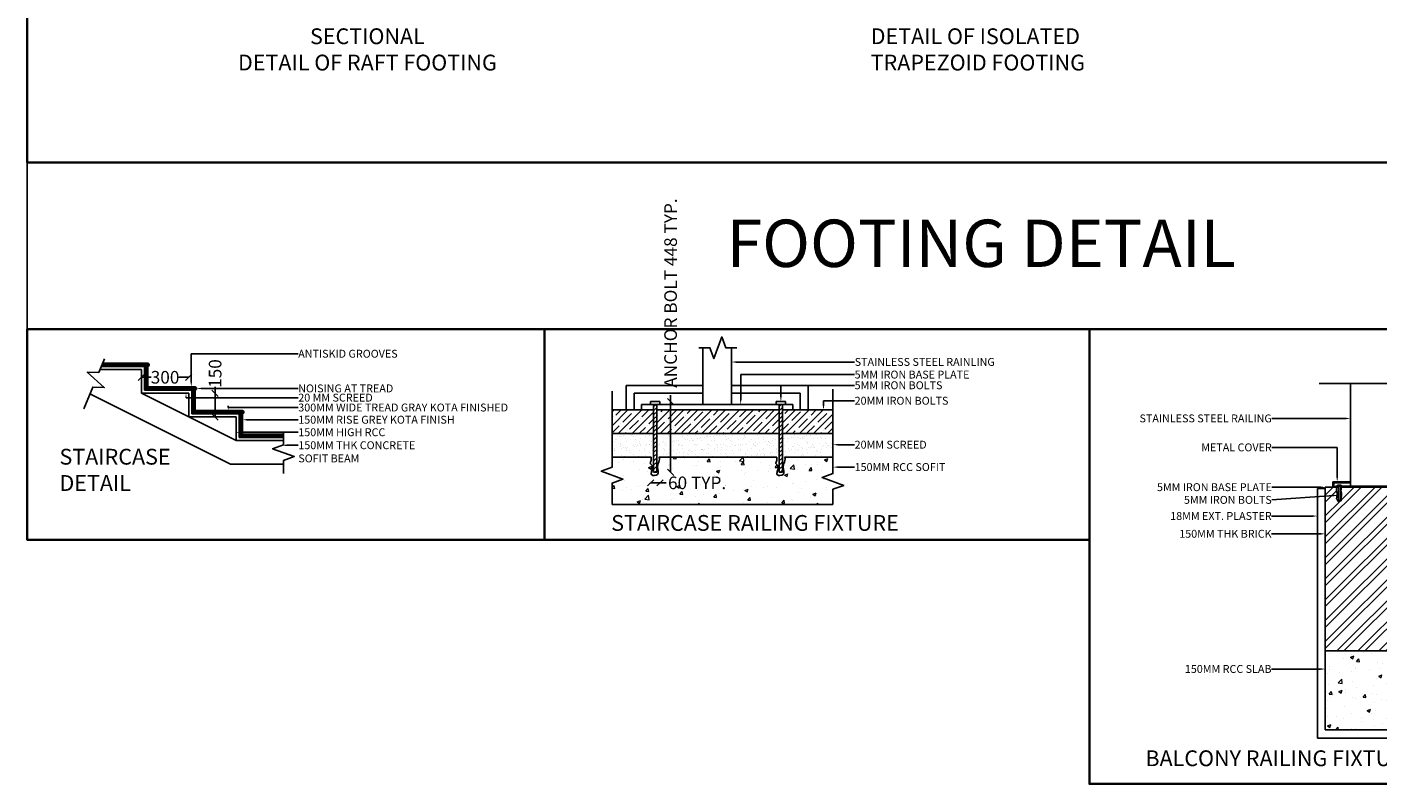
# Model space of a CAD drawing. Units: millimetres. Extents: x -6233 to 6805, y -5269 to 4890.
# Tile 1 of 4: x -6233 to 2321, y -5269 to -472. Entities that reach past the tile are written whole.
import ezdxf
from ezdxf import colors
from ezdxf.entities.mleader import LeaderData, LeaderLine
from ezdxf.math import Vec2, Vec3

# ---------------------------------------------------------------- set-up
doc = ezdxf.new("R2010")
doc.units = ezdxf.units.MM
doc.header["$MEASUREMENT"] = 0
for name, color, linetype, lineweight in [('A-FLOR-HRAL', 4, 'Continuous', 25), ('A-FLOR-STRS', 7, 'Continuous', 25), ('S-ANNO-DIMS', 2, 'Continuous', 18), ('S-ANNO-TEXT', 3, 'Continuous', 18), ('S-ANNO-TTLB', 7, 'Continuous', 35), ('S-PATT', 252, 'Continuous', 13)]:
    doc.layers.add(name, color=color, linetype=linetype, lineweight=lineweight)
doc.styles.get("Standard").update_dxf_attribs({"font": 'arial.ttf'})
doc.dimstyles.get("Standard").update_dxf_attribs({"dimtxt": 80, "dimasz": 40, "dimexe": 0.18, "dimexo": 0.0625, "dimgap": 0.09, "dimtad": 0, "dimdec": 0, "dimzin": 0, "dimdsep": 46, "dimtxsty": 'Standard', "dimblk": 'OBLIQUE', "dimcen": 0.09, "dimadec": 0, "dimazin": 0, "dimtfac": 1, "dimtdec": 0, "dimtofl": 0, "dimtmove": 0, "dimatfit": 3, "dimfxl": 1, "dimfxlon": 1, "dimtolj": 1, "dimtzin": 0, "dimarcsym": 0})

# ---------------------------------------------------------------- blocks, each defined once
blk = doc.blocks.new('_Oblique')
at = {"color": 0, "linetype": 'ByBlock', "lineweight": -2}
blk.add_line((-0.5, -0.5), (0.5, 0.5), dxfattribs=at)
blk = doc.blocks.new('*D23')
at = {"layer": 'DEFPOINTS', "color": 0, "transparency": 16777216}
for p in [(-5208.1, -2691.9), (-5508.1, -2792.8), (-5208.1, -2792.8)]:
    blk.add_point(p, dxfattribs=at)
at = {"layer": 'S-ANNO-DIMS', "color": 0, "lineweight": -2, "transparency": 16777216}
for p, q in [((-5508.1, -2692.9), (-5508.1, -2691.7)), ((-5508.1, -2691.9), (-5446.4, -2691.9)), ((-5208.1, -2691.9), (-5269.8, -2691.9)), ((-5208.1, -2692.9), (-5208.1, -2691.7))]:
    blk.add_line(p, q, dxfattribs=at)
at = {"layer": 'S-ANNO-DIMS', "color": 0, "lineweight": -2, "transparency": 16777216, "xscale": 40, "yscale": 40, "zscale": 40, "rotation": 180}
blk.add_blockref('_Oblique', (-5508.1, -2691.9), dxfattribs=at)
at = {"layer": 'S-ANNO-DIMS', "color": 0, "lineweight": -2, "transparency": 16777216, "xscale": 40, "yscale": 40, "zscale": 40}
blk.add_blockref('_Oblique', (-5208.1, -2691.9), dxfattribs=at)
at = {"layer": 'S-ANNO-DIMS', "color": 0, "transparency": 16777216, "insert": (-5358.1, -2691.9), "char_height": 80, "attachment_point": 5}
blk.add_mtext('\\A1;300', dxfattribs=at)
blk = doc.blocks.new('*D24')
at = {"layer": 'DEFPOINTS', "color": 0, "transparency": 16777216}
for p in [(-5208.1, -2792.8), (-5040.8, -2792.8), (-5208.1, -2942.8)]:
    blk.add_point(p, dxfattribs=at)
at = {"layer": 'S-ANNO-DIMS', "color": 0, "lineweight": -2, "transparency": 16777216}
for p, q in [((-5041.8, -2792.8), (-5040.6, -2792.8)), ((-5040.8, -2792.8), (-5040.8, -2752.8)), ((-5040.8, -2942.8), (-5040.8, -2792.8)), ((-5041.8, -2942.8), (-5040.6, -2942.8))]:
    blk.add_line(p, q, dxfattribs=at)
at = {"layer": 'S-ANNO-DIMS', "color": 0, "lineweight": -2, "transparency": 16777216, "xscale": 40, "yscale": 40, "zscale": 40}
for p, rotation in [((-5040.8, -2792.8), 90), ((-5040.8, -2942.8), 270)]:
    blk.add_blockref('_Oblique', p, dxfattribs=dict(at, rotation=rotation))
at = {"layer": 'S-ANNO-DIMS', "color": 0, "transparency": 16777216, "insert": (-5040.8, -2668.2), "char_height": 80, "attachment_point": 5, "rotation": 90}
blk.add_mtext('\\A1;150', dxfattribs=at)
blk = doc.blocks.new('ANCHOR-BOLT-STAIR')
for p, q in [((0, 429.2), (0, 447.9)), ((0, 447.9), (59.9, 447.9)), ((19.4, 429.2), (0, 429.2)), ((19.4, 429.2), (19.4, 0)), ((39.4, 429.2), (39.4, 0)), ((59.9, 429.2), (39.4, 429.2)), ((59.9, 447.9), (59.9, 429.2)), ((39.4, 0), (19.4, 0))]:
    blk.add_line(p, q)
blk = doc.blocks.new('*D32')
at = {"layer": 'DEFPOINTS', "color": 0, "transparency": 16777216}
for p in [(-2222, -2845.6), (-2154.8, -2845.6), (-2222, -3293.5)]:
    blk.add_point(p, dxfattribs=at)
at = {"layer": 'S-ANNO-DIMS', "color": 0, "lineweight": -2, "transparency": 16777216}
for p, q in [((-2154.8, -2845.6), (-2154.8, -2805.6)), ((-2155.8, -2845.6), (-2154.7, -2845.6)), ((-2154.8, -3293.5), (-2154.8, -2845.6)), ((-2155.8, -3293.5), (-2154.7, -3293.5))]:
    blk.add_line(p, q, dxfattribs=at)
at = {"layer": 'S-ANNO-DIMS', "color": 0, "lineweight": -2, "transparency": 16777216, "xscale": 40, "yscale": 40, "zscale": 40}
for p, rotation in [((-2154.8, -2845.6), 90), ((-2154.8, -3293.5), 270)]:
    blk.add_blockref('_Oblique', p, dxfattribs=dict(at, rotation=rotation))
at = {"layer": 'S-ANNO-DIMS', "color": 0, "transparency": 16777216, "insert": (-2154.8, -2158.3), "char_height": 80, "attachment_point": 5, "rotation": 90}
blk.add_mtext('\\A1;ANCHOR BOLT 448 TYP.', dxfattribs=at)
blk = doc.blocks.new('*D33')
at = {"layer": 'DEFPOINTS', "color": 0, "transparency": 16777216}
for p in [(-2281.9, -3293.5), (-2222, -3293.5), (-2222, -3360.7)]:
    blk.add_point(p, dxfattribs=at)
at = {"layer": 'S-ANNO-DIMS', "color": 0, "lineweight": -2, "transparency": 16777216}
for p, q in [((-2281.9, -3359.7), (-2281.9, -3360.8)), ((-2281.9, -3360.7), (-2222, -3360.7)), ((-2222, -3359.7), (-2222, -3360.8)), ((-2222, -3360.7), (-2182, -3360.7))]:
    blk.add_line(p, q, dxfattribs=at)
at = {"layer": 'S-ANNO-DIMS', "color": 0, "lineweight": -2, "transparency": 16777216, "xscale": 40, "yscale": 40, "zscale": 40, "rotation": 180}
blk.add_blockref('_Oblique', (-2281.9, -3360.7), dxfattribs=at)
at = {"layer": 'S-ANNO-DIMS', "color": 0, "lineweight": -2, "transparency": 16777216, "xscale": 40, "yscale": 40, "zscale": 40}
blk.add_blockref('_Oblique', (-2222, -3360.7), dxfattribs=at)
at = {"layer": 'S-ANNO-DIMS', "color": 0, "transparency": 16777216, "insert": (-1987, -3360.7), "char_height": 80, "attachment_point": 5}
blk.add_mtext('\\A1;60 TYP.', dxfattribs=at)

msp = doc.modelspace()

# ---------------------------------------------------------------- hatches: boundary and pattern name
at = {"layer": 'S-PATT'}
h = msp.add_hatch(dxfattribs=at)
h.set_pattern_fill('ANSI31', color=256, scale=50)
h.set_pattern_definition([(45, (445.642, 4418.545), (-4.4194174, 4.4194174), [])])
h.paths.add_polyline_path([(-5468.1, -2602.8), (-5753.6, -2602.8), (-5761.9, -2622.8), (-5468.1, -2622.8, 1)])
h.paths.add_polyline_path([(-5468.1, -2622.8), (-5488.1, -2622.8), (-5488.1, -2772.8), (-5168.1, -2772.8, 1), (-5168.1, -2752.8), (-5468.1, -2752.8)])
h.paths.add_polyline_path([(-5168.1, -2772.8), (-5188.1, -2772.8), (-5188.1, -2922.8), (-4868.1, -2922.8, 1), (-4868.1, -2902.8), (-5168.1, -2902.8)])
h.paths.add_polyline_path([(-4868.1, -2922.8), (-4888.1, -2922.8), (-4888.1, -3072.8), (-4608.1, -3072.8), (-4608.1, -3052.8), (-4868.1, -3052.8)])
h = msp.add_hatch(dxfattribs=at)
h.set_pattern_fill('ANSI35', color=256, scale=250)
h.set_pattern_definition([(45, (1728.94, 2227.43), (-44.1942, 44.1942), []), (45, (1773.14, 2227.43), (-44.1942, 44.1942), [78.125, -15.625, 0, -15.625])])
h.paths.add_polyline_path([(-1466.5, -2898.6), (-2242.5, -2898.6), (-2242.5, -3048.6), (-1466.5, -3048.6)])
h.paths.add_polyline_path([(-1126.1, -2898.6), (-1446.5, -2898.6), (-1446.5, -3048.6), (-1126.1, -3048.6)])
h.paths.add_polyline_path([(-2262.5, -2898.6), (-2525.7, -2898.6), (-2525.7, -3048.6), (-2262.5, -3048.6)])
h = msp.add_hatch(dxfattribs=at)
h.set_pattern_fill('ANSI31', color=256, scale=150)
h.set_pattern_definition([(45, (1728.943, 2227.432), (-13.25825, 13.25825), [])])
h.paths.add_polyline_path([(-2242.5, -2864.2), (-2262.5, -2864.2), (-2262.5, -3293.5), (-2242.5, -3293.5)])
h.paths.add_polyline_path([(-1446.5, -2864.2), (-1466.5, -2864.2), (-1466.5, -3293.5), (-1446.5, -3293.5)])
h = msp.add_hatch(dxfattribs=at)
h.set_pattern_fill('AR-SAND', color=256, scale=30)
h.set_pattern_definition([(37.5, (1728.943, 2227.43), (-1.8898, 57.8047), [0, -45.6, 0, -51, 0, -48.75]), (7.5, (1728.94, 2227.43), (53.0933, 84.6644), [0, -24.6, 0, -41.1, 0, -15.75]), (327.5, (1692.043, 2227.43), (93.42426, 0.16977), [0, -15, 0, -54, 0, -70.5]), (317.5, (1692.04, 2227.43), (90.1838, 26.3303), [0, -7.5, 0, -35.4, 0, -40.5])])
edge = h.paths.add_edge_path()
edge.add_line((-1466.5, -3048.6), (-2242.5, -3048.6))
edge.add_line((-2242.5, -3048.6), (-2242.5, -3293.5))
edge.add_line((-2242.5, -3293.5), (-2262.5, -3293.5))
edge.add_line((-2262.5, -3293.5), (-2262.5, -3048.6))
edge.add_line((-2262.5, -3048.6), (-2525.7, -3048.6))
edge.add_line((-2525.7, -3048.6), (-2525.7, -3198.6))
edge.add_line((-2525.7, -3198.6), (-2278.6, -3198.6))
edge.add_spline(control_points=[(-2278.6, -3198.6), (-2277.5, -3205.6), (-2275.5, -3218.5), (-2288.7, -3238.2), (-2260.8, -3253.8), (-2274.9, -3281.2), (-2280.9, -3317.9), (-2219.2, -3315.1), (-2245.1, -3262.2), (-2230.5, -3234.1), (-2221.5, -3202.7), (-2229.8, -3198.6)], knot_values=[0, 0, 0, 0, 20.99677, 39.349881, 56.133346, 95.091284, 114.829491, 151.719513, 198.433264, 232.426652, 262.634584, 262.634584, 262.634584, 262.634584], degree=3, periodic=0)
edge.add_line((-2229.8, -3198.6), (-1482.5, -3198.6))
edge.add_spline(control_points=[(-1482.5, -3198.6), (-1481.5, -3205.6), (-1479.5, -3218.5), (-1492.6, -3238.2), (-1464.8, -3253.8), (-1478.9, -3281.2), (-1484.9, -3317.9), (-1423.2, -3315.1), (-1449.1, -3262.2), (-1434.4, -3234.1), (-1425.5, -3202.7), (-1433.8, -3198.6)], knot_values=[0, 0, 0, 0, 20.99677, 39.349881, 56.133346, 95.091284, 114.829491, 151.719513, 198.433264, 232.426652, 262.634584, 262.634584, 262.634584, 262.634584], degree=3, periodic=0)
edge.add_line((-1433.8, -3198.6), (-1126.1, -3198.6))
edge.add_line((-1126.1, -3198.6), (-1126.1, -3048.6))
edge.add_line((-1126.1, -3048.6), (-1446.5, -3048.6))
edge.add_line((-1446.5, -3048.6), (-1446.5, -3293.5))
edge.add_line((-1446.5, -3293.5), (-1466.5, -3293.5))
edge.add_line((-1466.5, -3293.5), (-1466.5, -3048.6))
h = msp.add_hatch(dxfattribs=at)
h.set_pattern_fill('AR-CONC', color=256, scale=30)
h.set_pattern_definition([(50, (1728.94, 2227.43), (215.178, -18.8256), [22.5, -247.5]), (355, (1728.94, 2227.43), (-41.6254, 225.6576), [18, -198]), (100.4514, (1746.87, 2225.86), (173.5527, 206.832), [19.122, -210.3426]), (46.184, (1728.94, 2287.43), (320.172, -49.656), [33.75, -371.25]), (96.6356, (1755.62, 2283.3), (280.399, 292.236), [28.683, -315.514]), (351.184, (1728.94, 2287.43), (280.399, 292.236), [27, -297]), (21, (1758.94, 2272.43), (179.072, -120.7857), [22.5, -247.5]), (326, (1758.94, 2272.43), (72.9946, 217.545), [18, -198]), (71.4514, (1773.87, 2262.37), (252.067, 96.7593), [19.122, -210.3426]), (37.5, (1728.94, 2227.43), (3.64796, 99.86816), [0, -195.6, 0, -201, 0, -198.75]), (7.5, (1728.94, 2227.43), (78.9209, 118.3235), [0, -114.6, 0, -191.1, 0, -75.75]), (327.5, (1662.04, 2227.43), (160.1467, -6.7665), [0, -75, 0, -234, 0, -310.5]), (317.5, (1632.04, 2227.43), (174.9559, 30.0315), [0, -97.5, 0, -155.4, 0, -220.5])])
edge = h.paths.add_edge_path()
edge.add_spline(control_points=[(-2229.8, -3198.6), (-2221.5, -3202.7), (-2230.5, -3234.1), (-2245.1, -3262.2), (-2219.2, -3315.1), (-2280.9, -3317.9), (-2274.9, -3281.2), (-2260.8, -3253.8), (-2288.7, -3238.2), (-2275.5, -3218.5), (-2277.5, -3205.6), (-2278.6, -3198.6)], knot_values=[0, 0, 0, 0, 30.207932, 64.20132, 110.915071, 147.805093, 167.5433, 206.501238, 223.284703, 241.637814, 262.634584, 262.634584, 262.634584, 262.634584], degree=3, periodic=0)
edge.add_line((-2278.6, -3198.6), (-2525.7, -3198.6))
edge.add_line((-2525.7, -3198.6), (-2525.7, -3262.3))
edge.add_line((-2525.7, -3262.3), (-2594.4, -3287.3))
edge.add_line((-2594.4, -3287.3), (-2457, -3337.3))
edge.add_line((-2457, -3337.3), (-2525.7, -3362.3))
edge.add_line((-2525.7, -3362.3), (-2525.7, -3498.6))
edge.add_line((-2525.7, -3498.6), (-1126.1, -3498.6))
edge.add_line((-1126.1, -3498.6), (-1126.1, -3401.8))
edge.add_line((-1126.1, -3401.8), (-1057.5, -3376.8))
edge.add_line((-1057.5, -3376.8), (-1194.8, -3326.8))
edge.add_line((-1194.8, -3326.8), (-1126.1, -3301.8))
edge.add_line((-1126.1, -3301.8), (-1126.1, -3198.6))
edge.add_line((-1126.1, -3198.6), (-1433.8, -3198.6))
edge.add_spline(control_points=[(-1433.8, -3198.6), (-1425.5, -3202.7), (-1434.4, -3234.1), (-1449.1, -3262.2), (-1423.2, -3315.1), (-1484.9, -3317.9), (-1478.9, -3281.2), (-1464.8, -3253.8), (-1492.6, -3238.2), (-1479.5, -3218.5), (-1481.5, -3205.6), (-1482.5, -3198.6)], knot_values=[0, 0, 0, 0, 30.207932, 64.20132, 110.915071, 147.805093, 167.5433, 206.501238, 223.284703, 241.637814, 262.634584, 262.634584, 262.634584, 262.634584], degree=3, periodic=0)
edge.add_line((-1482.5, -3198.6), (-2229.8, -3198.6))
h = msp.add_hatch(dxfattribs=at)
h.set_pattern_fill('ANSI32', color=256, scale=250)
h.set_pattern_definition([(45, (-403.88, 395.55), (-66.2913, 66.2913), []), (45, (-359.68, 395.55), (-66.2913, 66.2913), [])])
h.paths.add_polyline_path([(2555.6, -3388.6), (2479.2, -3388.6), (2475, -3412), (2479.2, -3425.9), (2479.2, -3442.8), (2477.2, -3451.1), (2477.2, -3475.2), (2457.7, -3479.6), (2450.6, -3467.1), (2447.4, -3461.6), (2448.4, -3451.9), (2451.4, -3421.4), (2447.5, -3414.8), (2447.5, -3401.8), (2448.7, -3388.6), (2096.7, -3388.6), (2092.6, -3412), (2096.7, -3425.9), (2096.7, -3442.8), (2094.8, -3451), (2094.8, -3475.2), (2075.3, -3479.6), (2068.2, -3467.1), (2065, -3461.6), (2065.9, -3451.9), (2069, -3421.4), (2065.1, -3414.8), (2065.1, -3401.8), (2066.2, -3388.6), (1993.8, -3388.6), (1993.8, -4425), (2555.6, -4425)])
h = msp.add_hatch(dxfattribs=at)
h.set_pattern_fill('AR-CONC', color=256, scale=30)
h.set_pattern_definition([(50, (-403.88, 395.55), (215.178, -18.8256), [22.5, -247.5]), (355, (-403.88, 395.55), (-41.6254, 225.658), [18, -198]), (100.4514, (-385.94, 393.99), (173.5527, 206.832), [19.122, -210.3426]), (46.184, (-403.88, 455.55), (320.172, -49.656), [33.75, -371.25]), (96.6356, (-377.2, 451.42), (280.399, 292.236), [28.683, -315.514]), (351.184, (-403.88, 455.55), (280.399, 292.236), [27, -297]), (21, (-373.88, 440.55), (179.072, -120.7857), [22.5, -247.5]), (326, (-373.88, 440.55), (72.9946, 217.545), [18, -198]), (71.4514, (-358.95, 430.49), (252.067, 96.7593), [19.122, -210.3426]), (37.5, (-403.88, 395.554), (3.648, 99.8682), [0, -195.6, 0, -201, 0, -198.75]), (7.5, (-403.88, 395.55), (78.9209, 118.3235), [0, -114.6, 0, -191.1, 0, -75.75]), (327.5, (-470.78, 395.55), (160.1467, -6.7665), [0, -75, 0, -234, 0, -310.5]), (317.5, (-500.78, 395.55), (174.9559, 30.0315), [0, -97.5, 0, -155.4, 0, -220.5])])
h.paths.add_polyline_path([(3117.4, -4925), (3117.4, -4675), (3460.8, -4550), (3117.4, -4425), (1993.8, -4425), (1993.8, -4925)])

# ---------------------------------------------------------------- linework, layer by layer
at = {"layer": 'A-FLOR-HRAL'}
for p, q in [((-1951, -2864.2), (-1951, -2505.1)), ((-1769.2, -2864.2), (-1769.2, -2505.1)), ((2153.7, -3388.6), (2153.7, -2730.5)), ((-2436, -2898.6), (-2436, -2743)), ((-2436, -2743), (-1951, -2743)), ((-2386, -2898.6), (-2386, -2793)), ((-2386, -2793), (-1951, -2793)), ((-1284.2, -2743), (-1769.2, -2743)), ((-1334.2, -2793), (-1769.2, -2793)), ((-1334.2, -2898.6), (-1334.2, -2793)), ((-1284.2, -2898.6), (-1284.2, -2743)), ((-2525.7, -2898.6), (-2262.5, -2898.6)), ((-2525.7, -2898.6), (-2262.5, -2898.6)), ((-1380.8, -2864.2), (-2339.4, -2864.2)), ((-2339.4, -2864.2), (-2339.4, -2898.6)), ((-2242.5, -2898.6), (-1466.5, -2898.6)), ((-2242.5, -2898.6), (-1466.5, -2898.6)), ((-1446.5, -2898.6), (-1126.1, -2898.6)), ((-1446.5, -2898.6), (-1126.1, -2898.6)), ((-1380.8, -2898.6), (-1380.8, -2864.2)), ((-2525.7, -3048.6), (-2262.5, -3048.6)), ((-2242.5, -3048.6), (-1466.5, -3048.6)), ((-1446.5, -3048.6), (-1126.1, -3048.6)), ((-2525.7, -3198.6), (-2278.6, -3198.6)), ((-2229.8, -3198.6), (-1482.5, -3198.6)), ((-1433.8, -3198.6), (-1126.1, -3198.6)), ((1993.8, -3397.4), (1943.8, -3397.4)), ((1943.8, -3397.4), (1943.8, -4979.4)), ((1993.8, -3388.6), (1993.8, -4925)), ((1993.8, -3388.6), (2077.2, -3388.6)), ((2077.2, -3388.6), (1993.8, -3388.6)), ((2042.3, -3388.6), (2042.3, -3355.2)), ((2042.3, -3355.2), (2153.7, -3355.2)), ((2048.2, -3388.6), (2048.2, -3359.8)), ((2048.2, -3359.8), (2153.7, -3359.8)), ((2486.4, -3382.1), (2057.2, -3382.1)), ((2057.2, -3382.1), (2057.2, -3388.6)), ((2066.2, -3388.6), (2065.1, -3401.8)), ((2065.1, -3401.8), (2065.1, -3414.8)), ((2065.1, -3414.8), (2069, -3421.4)), ((2069, -3421.4), (2065.9, -3451.9)), ((2094.2, -3376), (2071.7, -3376)), ((2071.7, -3376), (2071.7, -3382.1)), ((2071.7, -3382.1), (2075.5, -3382.1)), ((2088, -3382.1), (2075.5, -3382.1)), ((2077.2, -3382.1), (2077.2, -3472.8)), ((2088, -3382.1), (2094.2, -3382.1)), ((2089.6, -3472.8), (2089.6, -3382.1)), ((2089.6, -3388.6), (2459.7, -3388.6)), ((2459.7, -3388.6), (2089.6, -3388.6)), ((2092.6, -3412), (2096.7, -3388.6)), ((2096.7, -3425.9), (2092.6, -3412)), ((2094.2, -3382.1), (2094.2, -3376)), ((-2525.7, -3498.6), (-1126.1, -3498.6)), ((2065.9, -3451.9), (2065, -3461.6)), ((2065, -3461.6), (2068.2, -3467.1)), ((2068.2, -3467.1), (2075.3, -3479.6)), ((2075.3, -3479.6), (2094.8, -3475.2)), ((2077.2, -3472.8), (2089.6, -3472.8)), ((2094.8, -3450), (2096.7, -3442.8)), ((2094.8, -3475.2), (2094.8, -3450)), ((2096.7, -3442.8), (2096.7, -3425.9)), ((1993.8, -4425), (3117.4, -4425)), ((1993.8, -4925), (3117.4, -4925)), ((1943.8, -4979.4), (3117.4, -4979.4))]:
    msp.add_line(p, q, dxfattribs=at)
for points in [[(1954.9, -2730.5), (2467.4, -2730.5), (2592.4, -3073.9), (2842.4, -2387.1), (2967.4, -2730.5), (3126.4, -2730.5)], [(-1734.7, -2505.1), (-1805.6, -2505.1), (-1830.6, -2436.4), (-1880.6, -2573.8), (-1905.6, -2505.1), (-1976.5, -2505.1)], [(-2525.7, -2779.6), (-2525.7, -3262.3), (-2594.4, -3287.3), (-2457, -3337.3), (-2525.7, -3362.3), (-2525.7, -3498.8)], [(-1126.1, -2767.8), (-1126.1, -3301.8), (-1194.8, -3326.8), (-1057.5, -3376.8), (-1126.1, -3401.8), (-1126.1, -3498.8)]]:
    msp.add_lwpolyline(points, dxfattribs=at)
for points in [[(-2278.6, -3198.6), (-2277.5, -3205.6), (-2275.5, -3218.5), (-2288.7, -3238.2), (-2260.8, -3253.8), (-2274.9, -3281.2), (-2280.9, -3317.9), (-2219.2, -3315.1), (-2245.1, -3262.2), (-2230.5, -3234.1), (-2221.5, -3202.7), (-2229.8, -3198.6)], [(-1482.5, -3198.6), (-1481.5, -3205.6), (-1479.5, -3218.5), (-1492.6, -3238.2), (-1464.8, -3253.8), (-1478.9, -3281.2), (-1484.9, -3317.9), (-1423.2, -3315.1), (-1449.1, -3262.2), (-1434.4, -3234.1), (-1425.5, -3202.7), (-1433.8, -3198.6)]]:
    msp.add_open_spline(points, degree=3, knots=[0, 0, 0, 0, 20.99677, 39.349881, 56.133346, 95.091284, 114.829491, 151.719513, 198.433264, 232.426652, 262.634584, 262.634584, 262.634584, 262.634584], dxfattribs=at)
at = {"layer": 'A-FLOR-STRS'}
for p, q in [((-6232.9, -1330.2), (-6232.9, -2387.1)), ((-5508.1, -2642.8), (-5770.2, -2642.8)), ((-5468.1, -2622.8), (-5761.9, -2622.8)), ((-5468.1, -2602.8), (-5753.6, -2602.8)), ((-5508.1, -2792.8), (-5508.1, -2642.8)), ((-5488.1, -2772.8), (-5488.1, -2622.8)), ((-5468.1, -2752.8), (-5468.1, -2622.8)), ((-5834.2, -2797.5), (-4943.5, -3242.8)), ((-5208.1, -2792.8), (-5508.1, -2792.8)), ((-5508.1, -2792.8), (-4908.1, -3092.8)), ((-5168.1, -2772.8), (-5488.1, -2772.8)), ((-5168.1, -2752.8), (-5468.1, -2752.8)), ((-5208.1, -2942.8), (-5208.1, -2792.8)), ((-5188.1, -2922.8), (-5188.1, -2772.8)), ((-5168.1, -2902.8), (-5168.1, -2772.8)), ((-4868.1, -2902.8), (-5168.1, -2902.8)), ((-4908.1, -2942.8), (-5208.1, -2942.8)), ((-4868.1, -2922.8), (-5188.1, -2922.8)), ((-4908.1, -3092.8), (-4908.1, -2942.8)), ((-4888.1, -3072.8), (-4888.1, -2922.8)), ((-4868.1, -3052.8), (-4868.1, -2922.8)), ((-4608.1, -3072.8), (-4888.1, -3072.8)), ((-4608.1, -3052.8), (-4868.1, -3052.8)), ((-4608.1, -3092.8), (-4908.1, -3092.8)), ((-4608.1, -3092.8), (-4908.1, -3092.8)), ((-4908.1, -3242.8), (-4943.5, -3242.8)), ((-4608.1, -3242.8), (-4908.1, -3242.8))]:
    msp.add_line(p, q, dxfattribs=at)
for points in [[(-5742.3, -2575.4), (-5778.1, -2662), (-5851.2, -2658.8), (-5743.3, -2757.5), (-5816.4, -2754.4), (-5873.3, -2891.9)], [(-4608.1, -3037.8), (-4608.1, -3119.7), (-4676.8, -3144.7), (-4539.4, -3194.7), (-4608.1, -3219.7), (-4608.1, -3301.7)]]:
    msp.add_lwpolyline(points, dxfattribs=at)
for centre in [(-5468.1, -2612.8), (-5168.1, -2762.8), (-4868.1, -2912.8)]:
    msp.add_arc(centre, 10, 270, 90, dxfattribs=at)
at = {"layer": 'S-ANNO-TTLB'}
msp.add_line((-6232.9, -2387.1), (6804.5, -2387.1), dxfattribs=at)
for points in [[(-6232.9, 4890.2), (2600.5, 4890.2), (2600.5, -1330.2), (-6232.9, -1330.2)], [(-6232.9, -2387.1), (-2954.4, -2387.1), (-2954.4, -3721.1), (-6232.9, -3721.1)], [(-2954.4, -2387.1), (499.3, -2387.1), (499.3, -3721.1), (-2954.4, -3721.1)], [(499.3, -2387.1), (3596.8, -2387.1), (3596.8, -5268.9), (499.3, -5268.9)]]:
    msp.add_lwpolyline(points, close=True, dxfattribs=at)

# ---------------------------------------------------------------- block references
at = {"layer": 'A-FLOR-HRAL'}
for p in [(-2281.9, -3293.5), (-1485.9, -3293.5)]:
    msp.add_blockref('ANCHOR-BOLT-STAIR', p, dxfattribs=at)

# ---------------------------------------------------------------- texts
at = {"layer": 'S-ANNO-TEXT', "attachment_point": 1}
for s, width, insert, char_height in [('\\pxqc;SECTIONAL\\PDETAIL OF RAFT FOOTING', 1812.356, (-4982.2, -481.1), 100), ('DETAIL OF ISOLATED\\PTRAPEZOID FOOTING', 1812.356, (-887, -481.1), 100), ('{\\fArial|b1|i0|c0|p34;FOOTING DETAIL}', 3747.332, (-1800.8, -1693.1), 300), ('STAIRCASE\\PDETAIL', 915.26, (-6027.2, -3145.2), 100), ('STAIRCASE RAILING FIXTURE', 2161.186, (-2531.3, -3564.8), 100), ('BALCONY RAILING FIXTURE', 2161.186, (853.7, -5055.9), 100)]:
    msp.add_mtext_dynamic_manual_height_columns(s, width=width, gutter_width=1, heights=[0], dxfattribs=dict(at, insert=insert, char_height=char_height))

# ---------------------------------------------------------------- dimensions: what is measured, and where the dimension line sits
at = {"layer": 'S-ANNO-DIMS'}
dim = msp.add_linear_dim(base=(-2154.8, -2845.6), p1=(-2222, -3293.5), p2=(-2222, -2845.6), angle=90, text='ANCHOR BOLT <> TYP.', dimstyle='Standard', override={"dimdec": 0, "dimrnd": 0, "dimzin": 0, "dimlunit": 2}, dxfattribs=at)
dim.commit()
dim.dimension.update_dxf_attribs({"geometry": '*D32', "text_midpoint": (-2154.8, -2158.3)})
dim = msp.add_linear_dim(base=(-5040.8, -2792.8), p1=(-5208.1, -2942.8), p2=(-5208.1, -2792.8), angle=90, dimstyle='Standard', override={"dimclrd": 0, "dimclre": 0, "dimclrt": 0}, dxfattribs=at)
dim.commit()
dim.dimension.update_dxf_attribs({"geometry": '*D24', "text_midpoint": (-5040.8, -2668.2)})
dim = msp.add_linear_dim(base=(-5208.1, -2691.9), p1=(-5508.1, -2792.8), p2=(-5208.1, -2792.8), dimstyle='Standard', override={"dimclrd": 0, "dimclre": 0, "dimclrt": 0}, dxfattribs=at)
dim.commit()
dim.dimension.update_dxf_attribs({"geometry": '*D23', "text_midpoint": (-5358.1, -2691.9)})
dim = msp.add_linear_dim(base=(-2222, -3360.7), p1=(-2281.9, -3293.5), p2=(-2222, -3293.5), text='<> TYP.', dimstyle='Standard', override={"dimdec": 0, "dimrnd": 0, "dimzin": 0, "dimlunit": 2}, dxfattribs=at)
dim.commit()
dim.dimension.update_dxf_attribs({"geometry": '*D33', "text_midpoint": (-1987, -3360.7)})

# ---------------------------------------------------------------- leaders
at = {"layer": 'S-ANNO-TEXT'}
ml = msp.add_multileader_mtext('Standard', dxfattribs=at)
ml.set_content('ANTISKID GROOVES', color=256)
ml.set_leader_properties()
ml.build(insert=Vec2(0, 0))
ml.multileader.update_dxf_attribs({"dogleg_length": 0.36, "arrow_head_size": 30})
ctx = ml.context
ctx.base_point, ctx.char_height, ctx.arrow_head_size, ctx.landing_gap_size, ctx.plane_origin = Vec3(-4514.6, -2543.1), 50, 30, 0.09, Vec3(-5192.1, -2752.8)
notes = []
notes.append((ctx, [(0, (1, 1, 0), (-4515, -2543.1), (1, 0), 0.36, [(0, [(-5192.1, -2752.8), (-5192.1, -2543.1)], 0, [])])]))
ctx.mtext.insert, ctx.mtext.flow_direction = Vec3(-4514.5, -2517.6), 5
ml = msp.add_multileader_mtext('Standard', dxfattribs=at)
ml.set_content('STAINLESS STEEL RAINLING', color=256)
ml.set_leader_properties()
ml.build(insert=Vec2(0, 0))
ml.multileader.update_dxf_attribs({"dogleg_length": 0.36, "arrow_head_size": 30})
ctx = ml.context
ctx.base_point, ctx.char_height, ctx.arrow_head_size, ctx.landing_gap_size, ctx.plane_origin = Vec3(-988.5, -2595.1), 50, 30, 0.09, Vec3(-1769.2, -2595.1)
notes.append((ctx, [(0, (1, 1, 0), (-988.9, -2595.1), (1, 0), 0.36, [(0, [(-1769.2, -2595.1)], 0, [])])]))
ctx.mtext.insert, ctx.mtext.flow_direction = Vec3(-988.4, -2569.6), 5
ml = msp.add_multileader_mtext('Standard', dxfattribs=at)
ml.set_content('5MM IRON BASE PLATE', color=256)
ml.set_leader_properties()
ml.build(insert=Vec2(0, 0))
ml.multileader.update_dxf_attribs({"dogleg_length": 0.36, "arrow_head_size": 30})
ctx = ml.context
ctx.base_point, ctx.char_height, ctx.arrow_head_size, ctx.landing_gap_size, ctx.plane_origin = Vec3(-988.9, -2675.2), 50, 30, 0.09, Vec3(-1710.8, -2864.2)
notes.append((ctx, [(0, (1, 1, 0), (-989.3, -2675.2), (1, 0), 0.36, [(0, [(-1710.8, -2864.2), (-1710.8, -2675.2)], 0, [])])]))
ctx.mtext.insert, ctx.mtext.flow_direction = Vec3(-988.9, -2649.8), 5
ml = msp.add_multileader_mtext('Standard', dxfattribs=at)
ml.set_content('NOISING AT TREAD', color=256)
ml.set_leader_properties()
ml.build(insert=Vec2(0, 0))
ml.multileader.update_dxf_attribs({"dogleg_length": 0.36, "arrow_head_size": 30})
ctx = ml.context
ctx.base_point, ctx.char_height, ctx.arrow_head_size, ctx.landing_gap_size, ctx.plane_origin = Vec3(-4514.6, -2762.8), 50, 30, 0.09, Vec3(-5158.1, -2762.8)
notes.append((ctx, [(0, (1, 1, 0), (-4515, -2762.8), (1, 0), 0.36, [(0, [(-5158.1, -2762.8)], 0, [])])]))
ctx.mtext.insert, ctx.mtext.flow_direction = Vec3(-4514.5, -2737.4), 5
ml = msp.add_multileader_mtext('Standard', dxfattribs=at)
ml.set_content('5MM IRON BOLTS ', color=256)
ml.set_leader_properties()
ml.build(insert=Vec2(0, 0))
ml.multileader.update_dxf_attribs({"dogleg_length": 0.36, "arrow_head_size": 30})
ctx = ml.context
ctx.base_point, ctx.char_height, ctx.arrow_head_size, ctx.landing_gap_size, ctx.plane_origin = Vec3(-988.9, -2743), 50, 30, 0.09, Vec3(-1456, -2845.6)
notes.append((ctx, [(0, (1, 1, 0), (-989.3, -2743), (1, 0), 0.36, [(0, [(-1456, -2845.6), (-1456, -2743)], 0, [])])]))
ctx.mtext.insert, ctx.mtext.flow_direction = Vec3(-988.9, -2717.6), 5
ml = msp.add_multileader_mtext('Standard', dxfattribs=at)
ml.set_content('20 MM SCREED', color=256)
ml.set_leader_properties()
ml.build(insert=Vec2(0, 0))
ml.multileader.update_dxf_attribs({"dogleg_length": 0.36, "arrow_head_size": 30})
ctx = ml.context
ctx.base_point, ctx.char_height, ctx.arrow_head_size, ctx.landing_gap_size, ctx.plane_origin = Vec3(-4514.2, -2821.4), 50, 30, 0.09, Vec3(-5225.4, -2792.8)
notes.append((ctx, [(0, (1, 1, 0), (-4514.6, -2821.4), (1, 0), 0.36, [(0, [(-5225.4, -2792.8), (-5225.4, -2821.4)], 0, [])])]))
ctx.mtext.insert, ctx.mtext.flow_direction = Vec3(-4514.1, -2795.9), 5
ml = msp.add_multileader_mtext('Standard', dxfattribs=at)
ml.set_content('20MM IRON BOLTS', color=256)
ml.set_leader_properties()
ml.build(insert=Vec2(0, 0))
ml.multileader.update_dxf_attribs({"dogleg_length": 0.36, "arrow_head_size": 30})
ctx = ml.context
ctx.base_point, ctx.char_height, ctx.arrow_head_size, ctx.landing_gap_size, ctx.plane_origin = Vec3(-988.9, -2840.9), 50, 30, 0.09, Vec3(-1186, -2898.6)
notes.append((ctx, [(0, (1, 1, 0), (-989.3, -2840.9), (1, 0), 0.36, [(0, [(-1186, -2898.6), (-1186, -2840.9)], 0, [])])]))
ctx.mtext.insert, ctx.mtext.flow_direction = Vec3(-988.9, -2815.5), 5
ml = msp.add_multileader_mtext('Standard', dxfattribs=at)
ml.set_content('300MM WIDE TREAD GRAY KOTA FINISHED', color=256)
ml.set_leader_properties()
ml.build(insert=Vec2(0, 0))
ml.multileader.update_dxf_attribs({"dogleg_length": 0.36, "arrow_head_size": 30})
ctx = ml.context
ctx.base_point, ctx.char_height, ctx.arrow_head_size, ctx.landing_gap_size, ctx.plane_origin = Vec3(-4514.2, -2884), 50, 30, 0.09, Vec3(-4958, -2902.8)
notes.append((ctx, [(0, (1, 1, 0), (-4514.6, -2884), (1, 0), 0.36, [(0, [(-4958, -2902.8), (-4958, -2884)], 0, [])])]))
ctx.mtext.insert, ctx.mtext.flow_direction = Vec3(-4514.1, -2858.5), 5
ml = msp.add_multileader_mtext('Standard', dxfattribs=at)
ml.set_content('150MM RISE GREY KOTA FINISH', color=256)
ml.set_leader_properties()
ml.build(insert=Vec2(0, 0))
ml.multileader.update_dxf_attribs({"dogleg_length": 0.36, "arrow_head_size": 30})
ctx = ml.context
ctx.base_point, ctx.char_height, ctx.arrow_head_size, ctx.landing_gap_size, ctx.plane_origin = Vec3(-4514.2, -2961.2), 50, 30, 0.09, Vec3(-4868.1, -2961.2)
notes.append((ctx, [(0, (1, 1, 0), (-4514.6, -2961.2), (1, 0), 0.36, [(0, [(-4868.1, -2961.2)], 0, [])])]))
ctx.mtext.insert, ctx.mtext.flow_direction = Vec3(-4514.1, -2935.8), 5
ml = msp.add_multileader_mtext('Standard', dxfattribs=at)
ml.set_content('STAINLESS STEEL RAILING   ', color=256)
ml.set_leader_properties()
ml.build(insert=Vec2(0, 0))
ml.multileader.update_dxf_attribs({"dogleg_length": 0.36, "arrow_head_size": 30})
ctx = ml.context
ctx.base_point, ctx.char_height, ctx.arrow_head_size, ctx.landing_gap_size, ctx.plane_origin = Vec3(738.3, -2952.9), 50, 30, 0.09, Vec3(2153.7, -2952.9)
ctx.text_align_type = 2
notes.append((ctx, [(0, (1, 1, 0), (1655.2, -2952.9), (-1, 0), 0.36, [(0, [(2153.7, -2952.9)], 0, [])])]))
ctx.mtext.insert, ctx.mtext.alignment, ctx.mtext.flow_direction = Vec3(1654.7, -2927.4), 3, 5
ml = msp.add_multileader_mtext('Standard', dxfattribs=at)
ml.set_content('150MM HIGH RCC', color=256)
ml.set_leader_properties()
ml.build(insert=Vec2(0, 0))
ml.multileader.update_dxf_attribs({"dogleg_length": 0.36, "arrow_head_size": 30})
ctx = ml.context
ctx.base_point, ctx.char_height, ctx.arrow_head_size, ctx.landing_gap_size, ctx.plane_origin = Vec3(-4514.2, -3040.7), 50, 30, 0.09, Vec3(-4908.1, -3040.7)
notes.append((ctx, [(0, (1, 1, 0), (-4514.6, -3040.7), (1, 0), 0.36, [(0, [(-4908.1, -3040.7)], 0, [])])]))
ctx.mtext.insert, ctx.mtext.flow_direction = Vec3(-4514.1, -3015.3), 5
ml = msp.add_multileader_mtext('Standard', dxfattribs=at)
ml.set_content('150MM THK CONCRETE\\PSOFIT BEAM', color=256)
ml.set_leader_properties()
ml.build(insert=Vec2(0, 0))
ml.multileader.update_dxf_attribs({"dogleg_length": 0.36, "arrow_head_size": 30})
ctx = ml.context
ctx.base_point, ctx.char_height, ctx.arrow_head_size, ctx.landing_gap_size, ctx.plane_origin = Vec3(-4513.9, -3123), 50, 30, 0.09, Vec3(-4617, -3123)
notes.append((ctx, [(0, (1, 1, 0), (-4514.2, -3123), (1, 0), 0.36, [(0, [(-4617, -3123)], 0, [])])]))
ctx.mtext.insert, ctx.mtext.flow_direction = Vec3(-4513.8, -3097.5), 5
ml = msp.add_multileader_mtext('Standard', dxfattribs=at)
ml.set_content('20MM SCREED ', color=256)
ml.set_leader_properties()
ml.build(insert=Vec2(0, 0))
ml.multileader.update_dxf_attribs({"dogleg_length": 0.36, "arrow_head_size": 30})
ctx = ml.context
ctx.base_point, ctx.char_height, ctx.arrow_head_size, ctx.landing_gap_size, ctx.plane_origin = Vec3(-988.9, -3119.3), 50, 30, 0.09, Vec3(-1126.1, -3119.3)
notes.append((ctx, [(0, (1, 1, 0), (-989.3, -3119.3), (1, 0), 0.36, [(0, [(-1126.1, -3119.3)], 0, [])])]))
ctx.mtext.insert, ctx.mtext.flow_direction = Vec3(-988.9, -3093.9), 5
ml = msp.add_multileader_mtext('Standard', dxfattribs=at)
ml.set_content('METAL COVER', color=256)
ml.set_leader_properties()
ml.build(insert=Vec2(0, 0))
ml.multileader.update_dxf_attribs({"dogleg_length": 0.36, "arrow_head_size": 30})
ctx = ml.context
ctx.base_point, ctx.char_height, ctx.arrow_head_size, ctx.landing_gap_size, ctx.plane_origin = Vec3(1159.7, -3136.5), 50, 30, 0.09, Vec3(2069, -3355.2)
ctx.text_align_type = 2
notes.append((ctx, [(0, (1, 1, 0), (1654.8, -3136.5), (-1, 0), 0.36, [(0, [(2069, -3355.2), (2069, -3136.5)], 0, [])])]))
ctx.mtext.insert, ctx.mtext.alignment, ctx.mtext.flow_direction = Vec3(1654.4, -3111), 3, 5
ml = msp.add_multileader_mtext('Standard', dxfattribs=at)
ml.set_content('150MM RCC SOFIT', color=256)
ml.set_leader_properties()
ml.build(insert=Vec2(0, 0))
ml.multileader.update_dxf_attribs({"dogleg_length": 0.36, "arrow_head_size": 30})
ctx = ml.context
ctx.base_point, ctx.char_height, ctx.arrow_head_size, ctx.landing_gap_size, ctx.plane_origin = Vec3(-988.9, -3261.1), 50, 30, 0.09, Vec3(-1126.1, -3261.1)
notes.append((ctx, [(0, (1, 1, 0), (-989.3, -3261.1), (1, 0), 0.36, [(0, [(-1126.1, -3261.1)], 0, [])])]))
ctx.mtext.insert, ctx.mtext.flow_direction = Vec3(-988.9, -3235.7), 5
ml = msp.add_multileader_mtext('Standard', dxfattribs=at)
ml.set_content('5MM IRON BASE PLATE', color=256)
ml.set_leader_properties()
ml.build(insert=Vec2(0, 0))
ml.multileader.update_dxf_attribs({"dogleg_length": 0.36, "arrow_head_size": 30})
ctx = ml.context
ctx.base_point, ctx.char_height, ctx.arrow_head_size, ctx.landing_gap_size, ctx.plane_origin = Vec3(865.2, -3388.6), 50, 30, 0.09, Vec3(1993.8, -3388.6)
ctx.text_align_type = 2
notes.append((ctx, [(0, (1, 1, 0), (1654.8, -3388.6), (-1, 0), 0.36, [(0, [(1993.8, -3388.6)], 0, [])])]))
ctx.mtext.insert, ctx.mtext.alignment, ctx.mtext.flow_direction = Vec3(1654.4, -3363.2), 3, 5
ml = msp.add_multileader_mtext('Standard', dxfattribs=at)
ml.set_content('5MM IRON BOLTS', color=256)
ml.set_leader_properties()
ml.build(insert=Vec2(0, 0))
ml.multileader.update_dxf_attribs({"dogleg_length": 0.36, "arrow_head_size": 30})
ctx = ml.context
ctx.base_point, ctx.char_height, ctx.arrow_head_size, ctx.landing_gap_size, ctx.plane_origin = Vec3(1062.8, -3469.1), 50, 30, 0.09, Vec3(2077.2, -3439.1)
ctx.text_align_type = 2
notes.append((ctx, [(0, (1, 1, 0), (1654.5, -3469.1), (-1, 0), 0.36, [(0, [(2077.2, -3439.1)], 0, [])])]))
ctx.mtext.insert, ctx.mtext.alignment, ctx.mtext.flow_direction = Vec3(1654, -3443.7), 3, 5
ml = msp.add_multileader_mtext('Standard', dxfattribs=at)
ml.set_content('18MM EXT. PLASTER', color=256)
ml.set_leader_properties()
ml.build(insert=Vec2(0, 0))
ml.multileader.update_dxf_attribs({"dogleg_length": 0.36, "arrow_head_size": 30})
ctx = ml.context
ctx.base_point, ctx.char_height, ctx.arrow_head_size, ctx.landing_gap_size, ctx.plane_origin = Vec3(955.6, -3571.1), 50, 30, 0.09, Vec3(1943.8, -3571.1)
ctx.text_align_type = 2
notes.append((ctx, [(0, (1, 1, 0), (1654.1, -3571.1), (-1, 0), 0.36, [(0, [(1943.8, -3571.1)], 0, [])])]))
ctx.mtext.insert, ctx.mtext.alignment, ctx.mtext.flow_direction = Vec3(1653.7, -3545.7), 3, 5
ml = msp.add_multileader_mtext('Standard', dxfattribs=at)
ml.set_content('150MM THK BRICK', color=256)
ml.set_leader_properties()
ml.build(insert=Vec2(0, 0))
ml.multileader.update_dxf_attribs({"dogleg_length": 0.36, "arrow_head_size": 30})
ctx = ml.context
ctx.base_point, ctx.char_height, ctx.arrow_head_size, ctx.landing_gap_size, ctx.plane_origin = Vec3(1036.1, -3683.9), 50, 30, 0.09, Vec3(1993.8, -3683.9)
ctx.text_align_type = 2
notes.append((ctx, [(0, (1, 1, 0), (1653.8, -3683.9), (-1, 0), 0.36, [(0, [(1993.8, -3683.9)], 0, [])])]))
ctx.mtext.insert, ctx.mtext.alignment, ctx.mtext.flow_direction = Vec3(1653.3, -3658.5), 3, 5
ml = msp.add_multileader_mtext('Standard', dxfattribs=at)
ml.set_content('150MM RCC SLAB', color=256)
ml.set_leader_properties()
ml.build(insert=Vec2(0, 0))
ml.multileader.update_dxf_attribs({"dogleg_length": 0.36, "arrow_head_size": 30})
ctx = ml.context
ctx.base_point, ctx.char_height, ctx.arrow_head_size, ctx.landing_gap_size, ctx.plane_origin = Vec3(1062.5, -4540.6), 50, 30, 0.09, Vec3(1993.8, -4540.6)
ctx.text_align_type = 2
notes.append((ctx, [(0, (1, 1, 0), (1653.4, -4540.6), (-1, 0), 0.36, [(0, [(1993.8, -4540.6)], 0, [])])]))
ctx.mtext.insert, ctx.mtext.alignment, ctx.mtext.flow_direction = Vec3(1652.9, -4515.1), 3, 5
for ctx, leaders in notes:
    for number, flags, end, landing, length, lines in leaders:
        leader = LeaderData()
        leader.index, (leader.has_last_leader_line, leader.has_dogleg_vector, leader.attachment_direction) = number, flags
        leader.last_leader_point, leader.dogleg_vector, leader.dogleg_length = Vec3(end), Vec3(landing), length
        for number, points, colour, breaks in lines:
            line = LeaderLine()
            line.index, line.vertices, line.color, line.breaks = number, Vec3.list(points), colors.encode_raw_color(colour), breaks
            leader.lines.append(line)
        ctx.leaders.append(leader)

doc.saveas('drawing.dxf')
